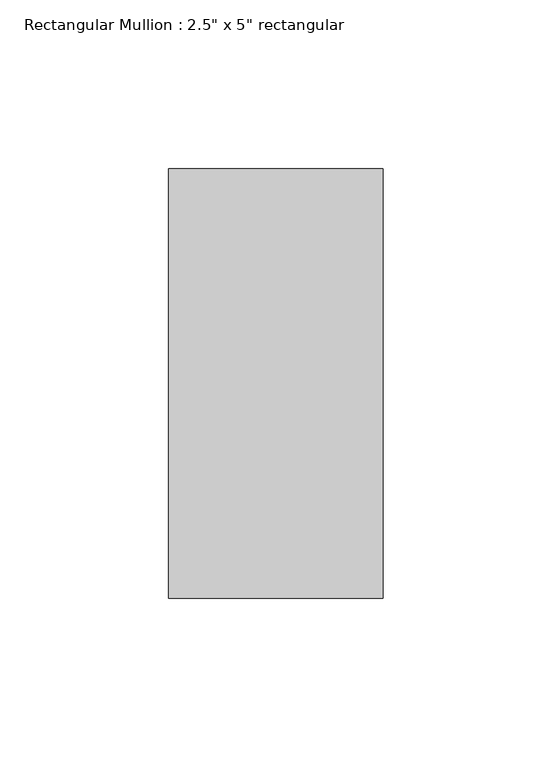
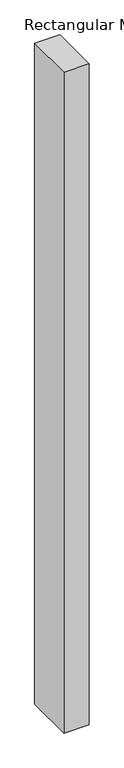
"""IFC4 building model written with IfcOpenShell, lengths in millimetres: member geometry."""

from ifc_helpers import new_model, si_unit, frame, origin, place, context, project, spatial, polyline, outline, extrude, source, transform, mapped, element, save


def member_3cb18284(model_context):
    return source(origin(), model_context, "Body", "SweptSolid", [
        extrude(outline(polyline([(0.0, 63.5), (0.0, -63.5), (-63.5, -63.5), (-63.5, 63.5), (0.0, 63.5)])), frame((0.0, 0.0, -1757.2747989), z_axis=(0.0, 0.0, 1.0), x_axis=(1.0, 0.0, 0.0)), (0.0, 0.0, 1.0), 1757.2747989),
    ])


if __name__ == "__main__":
    model = new_model("IFC4")
    model_context = context("Model", 3, world=origin())
    ifc_project = project(units=[si_unit("LENGTHUNIT", "METRE", prefix="MILLI")], contexts=[model_context])
    site = spatial("IfcSite", under=ifc_project)
    building = spatial("IfcBuilding", under=site)
    placement = place(None, origin())
    member_shape = member_3cb18284(model_context)
    element("IfcMember", 1, ObjectType="Rectangular Mullion : 2.5\" x 5\" rectangular", at=placement, inside=building, context=model_context, shape_type="MappedRepresentation", body=[
        mapped(member_shape, transform((0.0, 0.0, 0.0), x_axis=(1.0, 0.0, 0.0), y_axis=(0.0, 1.0, 0.0), z_axis=(0.0, 0.0, 1.0))),
    ])
    save(model, "model.ifc")

# Revit data of these elements
# Type "Rectangular Mullion : 2.5\" x 5\" rectangular"
#   built-in parameter 1007304 = 0.416667 (stored number, unit not read)
#   built-in parameter 1007301 = 0.104167 (stored number, unit not read)
#   built-in parameter 1007300 = 0.104167 (stored number, unit not read)
# Element 1 (IfcMember, "Rectangular Mullion : 2.5\" x 5\" rectangular")
#   Materials on its faces: "Aluminum"
# Materials
#   "Aluminum": class "Metal", colour RGB 247 247 247, transparency 0, Description = "Aluminum 6061", Cost = 0
